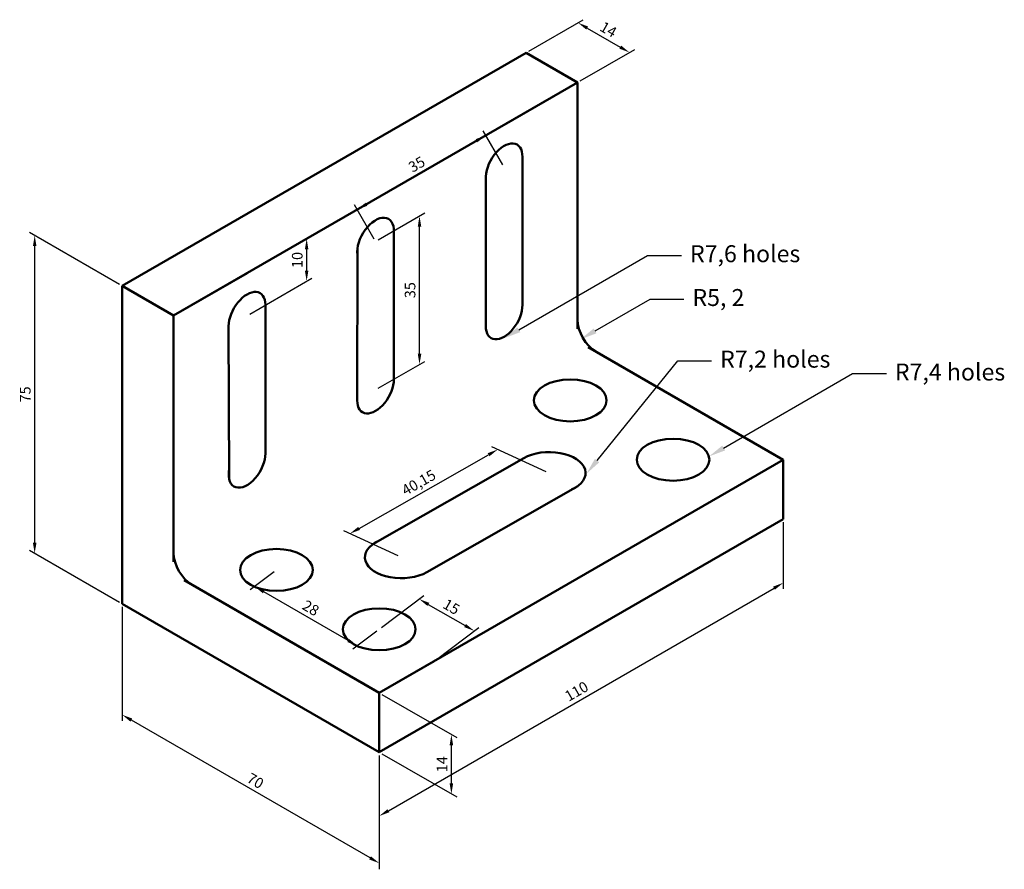
# Model space of a CAD drawing. Units: millimetres. Extents: x 4079 to 4311, y 953 to 1153.
import ezdxf
from ezdxf import colors
from ezdxf.entities.mleader import LeaderData, LeaderLine
from ezdxf.math import Vec2, Vec3

# ---------------------------------------------------------------- set-up
doc = ezdxf.new("R2010")
doc.units = ezdxf.units.MM
for name, color, linetype, lineweight in [('M-DIMS', 2, 'Continuous', 25), ('M-OUTL', 7, 'Continuous', 50), ('M-TEXT', 3, 'Continuous', 25)]:
    doc.layers.add(name, color=color, linetype=linetype, lineweight=lineweight)
doc.styles.get("Standard").update_dxf_attribs({"font": 'arial.ttf'})
doc.dimstyles.new('ISO-25', dxfattribs={"dimtxt": 2.5, "dimasz": 2.5, "dimexe": 1.25, "dimexo": 0.625, "dimtad": 1, "dimtxsty": 'Standard', "dimcen": 2.5, "dimadec": 0, "dimazin": 0, "dimtfac": 1, "dimtmove": 0, "dimatfit": 3, "dimfxl": 1, "dimarcsym": 0})

# ---------------------------------------------------------------- blocks, each defined once
blk = doc.blocks.new('*D1')
at = {"layer": 'Defpoints', "color": 0, "transparency": 16777216}
for p in [(4258.85, 1035.16), (4258.85, 1020.13), (4163.58, 980.16)]:
    blk.add_point(p, dxfattribs=at)
at = {"layer": 'M-DIMS', "color": 0, "lineweight": -2, "transparency": 16777216}
for p, q in [((4258.85, 1034.44), (4258.85, 1018.68)), ((4165.75, 966.38), (4256.68, 1018.88)), ((4163.58, 979.44), (4163.58, 963.68))]:
    blk.add_line(p, q, dxfattribs=at)
at = {"layer": 'M-DIMS', "color": 0, "transparency": 16777216}
for points in [[(4256.47, 1019.24), (4256.89, 1018.52), (4258.85, 1020.13)], [(4165.54, 966.74), (4165.96, 966.02), (4163.58, 965.13)]]:
    blk.add_solid(points, dxfattribs=at)
at = {"layer": 'M-DIMS', "color": 0, "transparency": 16777216, "insert": (4210.26, 994.27), "char_height": 2.5, "attachment_point": 5, "rotation": 30}
blk.add_mtext('110', dxfattribs=at)
blk = doc.blocks.new('*D2')
at = {"layer": 'Defpoints', "color": 0, "transparency": 16777216}
for p in [(4163.58, 994.16), (4180.6, 984.34), (4163.58, 980.16)]:
    blk.add_point(p, dxfattribs=at)
at = {"layer": 'M-DIMS', "color": 0, "lineweight": -2, "transparency": 16777216}
for p, q in [((4164.21, 993.8), (4181.85, 983.62)), ((4180.6, 972.84), (4180.6, 981.84)), ((4164.21, 979.8), (4181.85, 969.62))]:
    blk.add_line(p, q, dxfattribs=at)
at = {"layer": 'M-DIMS', "color": 0, "transparency": 16777216}
for points in [[(4180.18, 981.84), (4181.01, 981.84), (4180.6, 984.34)], [(4180.18, 972.84), (4181.01, 972.84), (4180.6, 970.34)]]:
    blk.add_solid(points, dxfattribs=at)
at = {"layer": 'M-DIMS', "color": 0, "transparency": 16777216, "insert": (4178.72, 977.34), "char_height": 2.5, "attachment_point": 5, "rotation": 90}
blk.add_mtext('14', dxfattribs=at)
blk = doc.blocks.new('*D3')
at = {"layer": 'Defpoints', "color": 0, "transparency": 16777216}
for p in [(4102.96, 1015.16), (4102.96, 989.01), (4163.58, 980.16)]:
    blk.add_point(p, dxfattribs=at)
at = {"layer": 'M-DIMS', "color": 0, "lineweight": -2, "transparency": 16777216}
for p, q in [((4102.96, 1014.44), (4102.96, 987.56)), ((4161.42, 955.26), (4105.13, 987.76)), ((4163.58, 979.44), (4163.58, 952.56))]:
    blk.add_line(p, q, dxfattribs=at)
at = {"layer": 'M-DIMS', "color": 0, "transparency": 16777216}
for points in [[(4105.33, 988.12), (4104.92, 987.39), (4102.96, 989.01)], [(4161.63, 955.62), (4161.21, 954.89), (4163.58, 954.01)]]:
    blk.add_solid(points, dxfattribs=at)
at = {"layer": 'M-DIMS', "color": 0, "transparency": 16777216, "insert": (4134.22, 973.15), "char_height": 2.5, "attachment_point": 5, "rotation": 330}
blk.add_mtext('70', dxfattribs=at)
blk = doc.blocks.new('*D4')
at = {"layer": 'Defpoints', "color": 0, "transparency": 16777216}
for p in [(4082.33, 1102.07), (4102.96, 1090.16), (4102.96, 1015.16)]:
    blk.add_point(p, dxfattribs=at)
at = {"layer": 'M-DIMS', "color": 0, "lineweight": -2, "transparency": 16777216}
for p, q in [((4102.34, 1090.52), (4081.08, 1102.79)), ((4082.33, 1029.57), (4082.33, 1099.57)), ((4102.34, 1015.52), (4081.08, 1027.79))]:
    blk.add_line(p, q, dxfattribs=at)
at = {"layer": 'M-DIMS', "color": 0, "transparency": 16777216}
for points in [[(4081.92, 1099.57), (4082.75, 1099.57), (4082.33, 1102.07)], [(4081.92, 1029.57), (4082.75, 1029.57), (4082.33, 1027.07)]]:
    blk.add_solid(points, dxfattribs=at)
at = {"layer": 'M-DIMS', "color": 0, "transparency": 16777216, "insert": (4080.44, 1064.57), "char_height": 2.5, "attachment_point": 5, "rotation": 90}
blk.add_mtext('75', dxfattribs=at)
blk = doc.blocks.new('*D5')
at = {"layer": 'Defpoints', "color": 0, "transparency": 16777216}
for p in [(4146.47, 1101.28), (4132.41, 1093.16), (4132.41, 1083.16)]:
    blk.add_point(p, dxfattribs=at)
at = {"layer": 'M-DIMS', "color": 0, "lineweight": -2, "transparency": 16777216}
for p, q in [((4133.03, 1093.52), (4147.72, 1102)), ((4146.47, 1093.78), (4146.47, 1098.78)), ((4133.03, 1083.52), (4147.72, 1092))]:
    blk.add_line(p, q, dxfattribs=at)
at = {"layer": 'M-DIMS', "color": 0, "transparency": 16777216}
for points in [[(4146.05, 1098.78), (4146.88, 1098.78), (4146.47, 1101.28)], [(4146.05, 1093.78), (4146.88, 1093.78), (4146.47, 1091.28)]]:
    blk.add_solid(points, dxfattribs=at)
at = {"layer": 'M-DIMS', "color": 0, "transparency": 16777216, "insert": (4144.57, 1096.28), "char_height": 2.5, "attachment_point": 5, "rotation": 90}
blk.add_mtext('10', dxfattribs=at)
blk = doc.blocks.new('*D6')
at = {"layer": 'Defpoints', "color": 0, "transparency": 16777216}
for p in [(4198.22, 1145.16), (4222.58, 1145.23), (4210.35, 1138.16)]:
    blk.add_point(p, dxfattribs=at)
at = {"layer": 'M-DIMS', "color": 0, "lineweight": -2, "transparency": 16777216}
for p, q in [((4198.85, 1145.52), (4211.71, 1152.95)), ((4212.63, 1150.98), (4220.42, 1146.48)), ((4210.97, 1138.52), (4223.83, 1145.95))]:
    blk.add_line(p, q, dxfattribs=at)
at = {"layer": 'M-DIMS', "color": 0, "transparency": 16777216}
for points in [[(4212.83, 1151.34), (4212.42, 1150.62), (4210.46, 1152.23)], [(4220.63, 1146.84), (4220.21, 1146.12), (4222.58, 1145.23)]]:
    blk.add_solid(points, dxfattribs=at)
at = {"layer": 'M-DIMS', "color": 0, "transparency": 16777216, "insert": (4217.46, 1150.36), "char_height": 2.5, "attachment_point": 5, "rotation": 330}
blk.add_mtext('14', dxfattribs=at)
blk = doc.blocks.new('*D7')
at = {"layer": 'Defpoints', "color": 0, "transparency": 16777216}
for p in [(4193.03, 1118.16), (4158.39, 1108.16), (4162.72, 1100.66)]:
    blk.add_point(p, dxfattribs=at)
at = {"layer": 'M-DIMS', "color": 0, "lineweight": -2, "transparency": 16777216}
for p, q in [((4192.72, 1118.7), (4188.07, 1126.75)), ((4186.53, 1124.41), (4160.55, 1109.41)), ((4162.4, 1101.2), (4157.76, 1109.25))]:
    blk.add_line(p, q, dxfattribs=at)
at = {"layer": 'M-DIMS', "color": 0, "transparency": 16777216}
for points in [[(4186.32, 1124.77), (4186.74, 1124.05), (4188.7, 1125.66)], [(4160.34, 1109.77), (4160.76, 1109.05), (4158.39, 1108.16)]]:
    blk.add_solid(points, dxfattribs=at)
at = {"layer": 'M-DIMS', "color": 0, "transparency": 16777216, "insert": (4172.59, 1118.56), "char_height": 2.5, "attachment_point": 5, "rotation": 30}
blk.add_mtext('35', dxfattribs=at)
blk = doc.blocks.new('*D8')
at = {"layer": 'Defpoints', "color": 0, "transparency": 16777216}
for p in [(4191.55, 1051.59), (4203.67, 1046.02), (4168.78, 1026.16)]:
    blk.add_point(p, dxfattribs=at)
at = {"layer": 'M-DIMS', "color": 0, "lineweight": -2, "transparency": 16777216}
for p, q in [((4202.97, 1046.34), (4190.15, 1052.23)), ((4158.83, 1032.97), (4189.38, 1050.35)), ((4168.08, 1026.48), (4155.26, 1032.37))]:
    blk.add_line(p, q, dxfattribs=at)
at = {"layer": 'M-DIMS', "color": 0, "transparency": 16777216}
for points in [[(4189.17, 1050.71), (4189.58, 1049.99), (4191.55, 1051.59)], [(4158.63, 1033.33), (4159.04, 1032.61), (4156.66, 1031.73)]]:
    blk.add_solid(points, dxfattribs=at)
at = {"layer": 'M-DIMS', "color": 0, "transparency": 16777216, "insert": (4173.05, 1043.51), "char_height": 2.5, "attachment_point": 5, "rotation": 29.6416}
blk.add_mtext('40,15', dxfattribs=at)
blk = doc.blocks.new('*D9')
at = {"layer": 'Defpoints', "color": 0, "transparency": 16777216}
for p in [(4163.58, 1009.16), (4185.99, 1008.8), (4176.57, 1001.66)]:
    blk.add_point(p, dxfattribs=at)
at = {"layer": 'M-DIMS', "color": 0, "lineweight": -2, "transparency": 16777216}
for p, q in [((4164.12, 1009.57), (4174.08, 1017.12)), ((4175.16, 1015.05), (4183.82, 1010.05)), ((4177.11, 1002.07), (4187.07, 1009.62))]:
    blk.add_line(p, q, dxfattribs=at)
at = {"layer": 'M-DIMS', "color": 0, "transparency": 16777216}
for points in [[(4175.37, 1015.41), (4174.95, 1014.69), (4173, 1016.3)], [(4184.03, 1010.41), (4183.61, 1009.69), (4185.99, 1008.8)]]:
    blk.add_solid(points, dxfattribs=at)
at = {"layer": 'M-DIMS', "color": 0, "transparency": 16777216, "insert": (4180.44, 1014.2), "char_height": 2.5, "attachment_point": 5, "rotation": 330}
blk.add_mtext('15', dxfattribs=at)
blk = doc.blocks.new('*D10')
at = {"layer": 'Defpoints', "color": 0, "transparency": 16777216}
for p in [(4139.33, 1023.16), (4134.2, 1019.27), (4163.58, 1009.16)]:
    blk.add_point(p, dxfattribs=at)
at = {"layer": 'M-DIMS', "color": 0, "lineweight": -2, "transparency": 16777216}
for p, q in [((4138.79, 1022.75), (4133.12, 1018.45)), ((4156.28, 1006.52), (4136.37, 1018.02)), ((4163.04, 1008.75), (4157.37, 1004.45))]:
    blk.add_line(p, q, dxfattribs=at)
at = {"layer": 'M-DIMS', "color": 0, "transparency": 16777216}
for points in [[(4136.57, 1018.38), (4136.16, 1017.66), (4134.2, 1019.27)], [(4156.49, 1006.88), (4156.08, 1006.16), (4158.45, 1005.27)]]:
    blk.add_solid(points, dxfattribs=at)
at = {"layer": 'M-DIMS', "color": 0, "transparency": 16777216, "insert": (4147.28, 1013.92), "char_height": 2.5, "attachment_point": 5, "rotation": 330}
blk.add_mtext('28', dxfattribs=at)
blk = doc.blocks.new('*D11')
at = {"layer": 'Defpoints', "color": 0, "transparency": 16777216}
for p in [(4173.08, 1106.65), (4162.72, 1100.66), (4162.72, 1065.66)]:
    blk.add_point(p, dxfattribs=at)
at = {"layer": 'M-DIMS', "color": 0, "lineweight": -2, "transparency": 16777216}
for p, q in [((4163.34, 1101.02), (4174.33, 1107.37)), ((4173.08, 1074.15), (4173.08, 1104.15)), ((4163.34, 1066.02), (4174.33, 1072.37))]:
    blk.add_line(p, q, dxfattribs=at)
at = {"layer": 'M-DIMS', "color": 0, "transparency": 16777216}
for points in [[(4172.67, 1104.15), (4173.5, 1104.15), (4173.08, 1106.65)], [(4172.67, 1074.15), (4173.5, 1074.15), (4173.08, 1071.65)]]:
    blk.add_solid(points, dxfattribs=at)
at = {"layer": 'M-DIMS', "color": 0, "transparency": 16777216, "insert": (4171.18, 1089.15), "char_height": 2.5, "attachment_point": 5, "rotation": 90}
blk.add_mtext('35', dxfattribs=at)

msp = doc.modelspace()

# ---------------------------------------------------------------- linework, layer by layer
at = {"layer": 'M-OUTL'}
for p, q in [((4102.962, 1090.163), (4198.224, 1145.163)), ((4198.224, 1145.163), (4210.349, 1138.163)), ((4115.086, 1083.163), (4210.349, 1138.163)), ((4210.349, 1138.163), (4193.028, 1128.163)), ((4210.349, 1138.163), (4210.349, 1080.05)), ((4197.358, 1120.731), (4197.358, 1085.663)), ((4188.709, 1116.024), (4188.698, 1080.665)), ((4167.044, 1103.371), (4167.047, 1068.164)), ((4158.427, 1098.865), (4158.387, 1063.17)), ((4115.086, 1083.163), (4132.406, 1093.163)), ((4102.962, 1015.163), (4102.962, 1090.163)), ((4102.962, 1090.163), (4115.086, 1083.163)), ((4136.737, 1085.663), (4136.737, 1050.663)), ((4115.086, 1083.163), (4115.086, 1025.05)), ((4128.156, 1044.755), (4128.076, 1080.65)), ((4258.846, 1049.163), (4212.849, 1075.72)), ((4162.08, 1029.252), (4197.646, 1049.539)), ((4163.583, 994.163), (4258.846, 1049.163)), ((4258.846, 1035.163), (4258.846, 1049.163)), ((4210.38, 1042.936), (4174.805, 1022.642)), ((4163.583, 980.163), (4258.846, 1035.163)), ((4163.583, 994.163), (4117.586, 1020.72)), ((4163.583, 980.163), (4102.962, 1015.163)), ((4163.583, 994.163), (4176.574, 1001.663)), ((4163.583, 994.163), (4159.253, 996.663)), ((4163.583, 980.163), (4163.583, 994.163))]:
    msp.add_line(p, q, dxfattribs=at)
for centre, major_axis, start_param, end_param in [((4193.028, 1118.163), (-3.062, -5.303), 2.3425609, 5.5681011), ((4162.717, 1100.663), (-3.062, -5.303), 2.3143532, 5.6314413), ((4132.406, 1083.163), (-3.062, -5.303), 2.3561945, 5.500343), ((4193.028, 1083.163), (-3.062, -5.303), 5.4974306, 8.6393931), ((4214.679, 1079.663), (-3.062, 5.303), 0.7853982, 2.3561945), ((4162.717, 1065.663), (-3.062, -5.303), 5.4964882, 8.6395056), ((4132.406, 1048.163), (-3.062, -5.303), 5.3108996, 8.6393798), ((4203.672, 1046.018), (-8.573, 0), 2.2309765, 5.4917447), ((4168.78, 1026.163), (-8.573, 0), 5.3741933, 8.6333717), ((4119.416, 1024.663), (-3.062, 5.303), 0.7853982, 2.3561945)]:
    msp.add_ellipse(centre, major_axis=major_axis, ratio=0.5773503, start_param=start_param, end_param=end_param, dxfattribs=at)
for centre in [(4208.617, 1063.163), (4232.865, 1049.163), (4139.335, 1023.163), (4163.583, 1009.163)]:
    msp.add_ellipse(centre, major_axis=(-8.573, 0), ratio=0.5773503, dxfattribs=at)

# ---------------------------------------------------------------- dimensions: what is measured, and where the dimension line sits
at = {"layer": 'M-DIMS'}
for p1, p2, distance, picture, middle in [((4198.224, 1145.163), (4210.349, 1138.163), 12.236, '*D6', (4217.463, 1150.356)), ((4193.028, 1118.163), (4162.717, 1100.663), -8.66, '*D7', (4172.592, 1118.561)), ((4162.717, 1065.663), (4162.717, 1100.663), -10.365, '*D11', (4171.18, 1089.148)), ((4102.962, 1015.163), (4102.962, 1090.163), 20.627, '*D4', (4080.438, 1064.572)), ((4132.406, 1083.163), (4132.406, 1093.163), -14.06, '*D5', (4144.565, 1096.281)), ((4168.78, 1026.163), (4203.672, 1046.018), 10.835, '*D8', (4173.053, 1043.509)), ((4163.583, 980.163), (4258.846, 1035.163), -13.021, '*D1', (4210.264, 994.274)), ((4163.583, 1009.163), (4139.335, 1023.163), 5.938, '*D10', (4147.276, 1013.918)), ((4163.583, 1009.163), (4176.574, 1001.663), 10.887, '*D9', (4180.443, 1014.196)), ((4163.583, 980.163), (4102.962, 1015.163), 22.653, '*D3', (4134.223, 973.152)), ((4163.583, 980.163), (4163.583, 994.163), -17.013, '*D2', (4178.716, 977.341))]:
    dim = msp.add_aligned_dim(p1=p1, p2=p2, distance=distance, dimstyle='ISO-25', override={"dimclrd": 0, "dimclre": 0, "dimclrt": 0}, dxfattribs=at)
    dim.commit()
    dim.dimension.update_dxf_attribs({"geometry": picture, "text_midpoint": middle})

# ---------------------------------------------------------------- leaders
at = {"layer": 'M-TEXT'}
ml = msp.add_multileader_mtext('Standard', dxfattribs=at)
ml.set_content('R7,6 holes ', color=256)
ml.set_leader_properties()
ml.build(insert=Vec2(0, 0))
ctx = ml.context
ctx.base_point, ctx.plane_origin = Vec3(4234.866, 1097.355), Vec3(4193.026, 1077.818)
notes = []
notes.append((ctx, [(0, (1, 1, 0), (4226.866, 1097.355), (1, 0), 8, [(0, [(4193.026, 1077.818)], 0, [])])]))
ctx.mtext.insert, ctx.mtext.flow_direction = Vec3(4236.866, 1099.751), 5
ml = msp.add_multileader_mtext('Standard', dxfattribs=at)
ml.set_content('R5, 2', color=256)
ml.set_leader_properties()
ml.build(insert=Vec2(0, 0))
ctx = ml.context
ctx.base_point, ctx.plane_origin = Vec3(4235.434, 1087.027), Vec3(4211.019, 1077.55)
notes.append((ctx, [(0, (1, 1, 0), (4227.434, 1087.027), (1, 0), 8, [(0, [(4211.019, 1077.55)], 0, [])])]))
ctx.mtext.insert, ctx.mtext.flow_direction = Vec3(4237.434, 1089.423), 5
ml = msp.add_multileader_mtext('Standard', dxfattribs=at)
ml.set_content('R7,2 holes ', color=256)
ml.set_leader_properties()
ml.build(insert=Vec2(0, 0))
ctx = ml.context
ctx.base_point, ctx.plane_origin = Vec3(4241.958, 1072.494), Vec3(4212.433, 1045.846)
notes.append((ctx, [(0, (1, 1, 0), (4233.958, 1072.494), (1, 0), 8, [(0, [(4212.433, 1045.846)], 0, [])])]))
ctx.mtext.insert, ctx.mtext.flow_direction = Vec3(4243.958, 1074.889), 5
ml = msp.add_multileader_mtext('Standard', dxfattribs=at)
ml.set_content('R7,4 holes ', color=256)
ml.set_leader_properties()
ml.build(insert=Vec2(0, 0))
ctx = ml.context
ctx.base_point, ctx.plane_origin = Vec3(4283.177, 1069.463), Vec3(4241.336, 1049.926)
notes.append((ctx, [(0, (1, 1, 0), (4275.177, 1069.463), (1, 0), 8, [(0, [(4241.336, 1049.926)], 0, [])])]))
ctx.mtext.insert, ctx.mtext.flow_direction = Vec3(4285.177, 1071.859), 5
for ctx, leaders in notes:
    for number, flags, end, landing, length, lines in leaders:
        leader = LeaderData()
        leader.index, (leader.has_last_leader_line, leader.has_dogleg_vector, leader.attachment_direction) = number, flags
        leader.last_leader_point, leader.dogleg_vector, leader.dogleg_length = Vec3(end), Vec3(landing), length
        for number, points, colour, breaks in lines:
            line = LeaderLine()
            line.index, line.vertices, line.color, line.breaks = number, Vec3.list(points), colors.encode_raw_color(colour), breaks
            leader.lines.append(line)
        ctx.leaders.append(leader)

doc.saveas('drawing.dxf')
